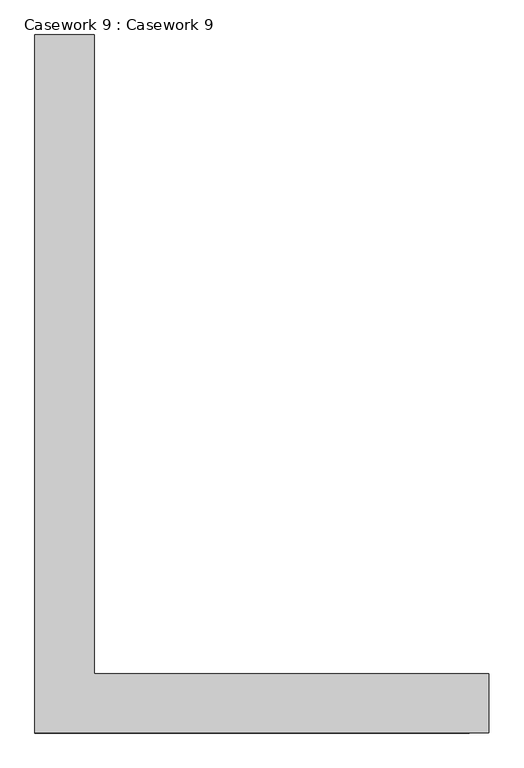
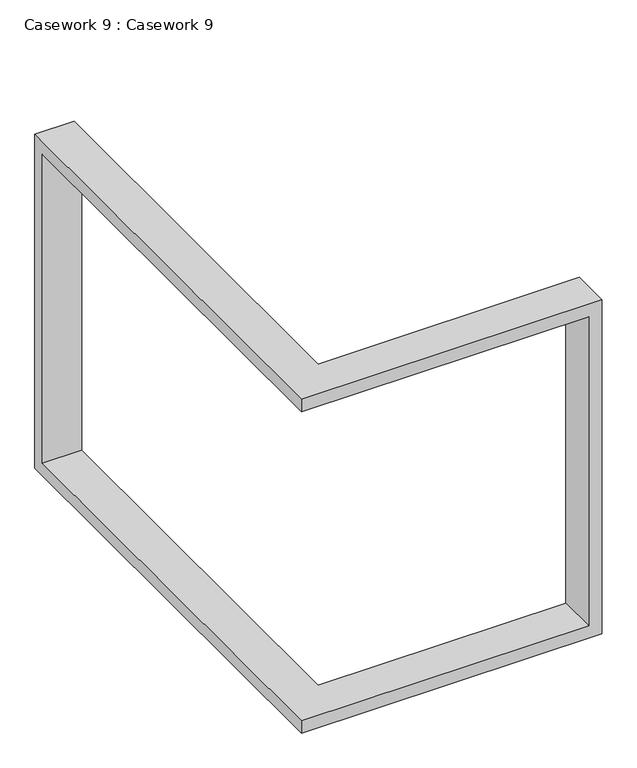
"""IFC4 building model written with IfcOpenShell, lengths in millimetres: furniture geometry, Casework 9 : Casework 9."""

from ifc_helpers import new_model, si_unit, origin, place, context, project, spatial, faceted_brep, source, transform, mapped, element, save


def casework_9_casework_9_0ee90f3f(model_context):
    return source(origin(), model_context, "Body", "Brep", [
        faceted_brep([(-6411.7953966, -7959.1929163, 3185.693809), (-6411.7953966, -11396.6929163, 3185.693809), (-6411.7953966, -11396.6929163, 3285.693809), (-6411.7953966, -7859.1929163, 3285.693809), (-6411.7953966, -7859.1929163, 585.693809), (-6411.7953966, -11396.6929163, 585.693809), (-6411.7953966, -11396.6929163, 685.693809), (-6411.7953966, -7959.1929163, 685.693809), (-6111.7953966, -7959.1929163, 3185.693809), (-6111.7953966, -7959.1929163, 685.693809), (-6111.7953966, -11096.6929163, 685.693809), (-6111.7953966, -11096.6929163, 585.693809), (-6111.7953966, -7859.1929163, 585.693809), (-6111.7953966, -7859.1929163, 3285.693809), (-6111.7953966, -11096.6929163, 3285.693809), (-6111.7953966, -11096.6929163, 3185.693809), (-4211.7953966, -11096.6929163, 3185.693809), (-4211.7953966, -11396.6929163, 3185.693809), (-4211.7953966, -11396.6929163, 685.693809), (-4111.7953966, -11396.6929163, 585.693809), (-4111.7953966, -11396.6929163, 3285.693809), (-4111.7953966, -11096.6929163, 3285.693809), (-4111.7953966, -11096.6929163, 585.693809), (-4211.7953966, -11096.6929163, 685.693809)], [[[0, 1, 2, 3, 4, 5, 6, 7]], [[8, 9, 10, 11, 12, 13, 14, 15]], [[0, 8, 15, 16, 17, 1]], [[2, 1, 17, 18, 6, 5, 19, 20]], [[2, 20, 21, 14, 13, 3]], [[4, 3, 13, 12]], [[4, 12, 11, 22, 19, 5]], [[6, 18, 23, 10, 9, 7]], [[0, 7, 9, 8]], [[21, 22, 11, 10, 23, 16, 15, 14]], [[18, 17, 16, 23]], [[20, 19, 22, 21]]]),
    ])


if __name__ == "__main__":
    model = new_model("IFC4")
    model_context = context("Model", 3, world=origin())
    ifc_project = project(units=[si_unit("LENGTHUNIT", "METRE", prefix="MILLI")], contexts=[model_context])
    site = spatial("IfcSite", under=ifc_project)
    building = spatial("IfcBuilding", under=site)
    placement = place(None, origin())
    casework_9_casework_9_shape = casework_9_casework_9_0ee90f3f(model_context)
    element("IfcFurniture", 1, ObjectType="Casework 9 : Casework 9", at=placement, inside=building, context=model_context, shape_type="MappedRepresentation", body=[
        mapped(casework_9_casework_9_shape, transform((0.0, 0.0, 0.0), x_axis=(1.0, 0.0, 0.0), y_axis=(0.0, 1.0, 0.0), z_axis=(0.0, 0.0, 1.0))),
    ])
    save(model, "model.ifc")
